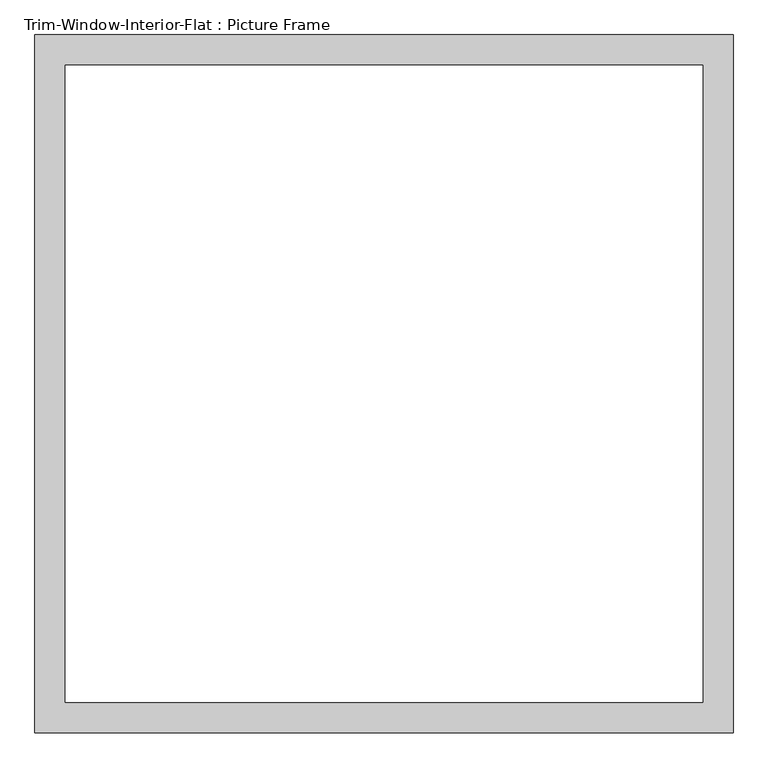
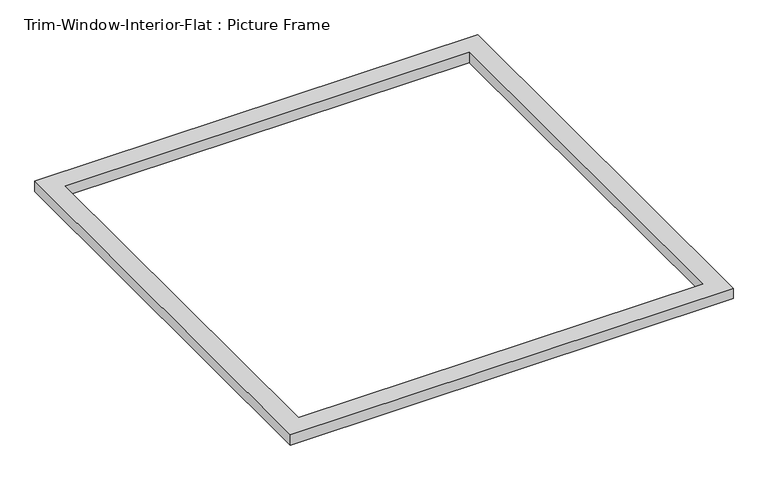
"""IFC4 building model written with IfcOpenShell, lengths in millimetres: proxy geometry, Trim-Window-Interior-Flat : Picture Frame."""

from ifc_helpers import new_model, si_unit, origin, origin_with_axes, place, context, project, spatial, polyline, outline, extrude, source, transform, mapped, element, save


def trim_window_interior_flat_picture_frame_caf2db4f(model_context):
    return source(origin(), model_context, "Body", "SweptSolid", [
        extrude(outline(polyline([(654.05, -44.45), (-654.05, -44.45), (-654.05, 1263.65), (654.05, 1263.65), (654.05, -44.45)]), holes=[polyline([(596.9, 12.7), (596.9, 1206.5), (-596.9, 1206.5), (-596.9, 12.7), (596.9, 12.7)])]), origin_with_axes(), (0.0, 0.0, 1.0), 31.75),
    ])


if __name__ == "__main__":
    model = new_model("IFC4")
    model_context = context("Model", 3, world=origin())
    ifc_project = project(units=[si_unit("LENGTHUNIT", "METRE", prefix="MILLI")], contexts=[model_context])
    site = spatial("IfcSite", under=ifc_project)
    building = spatial("IfcBuilding", under=site)
    placement = place(None, origin())
    trim_window_interior_flat_picture_frame_shape = trim_window_interior_flat_picture_frame_caf2db4f(model_context)
    element("IfcBuildingElementProxy", 1, Name="Trim-Window-Interior-Flat : Picture Frame", ObjectType="Trim-Window-Interior-Flat : Picture Frame", at=placement, inside=building, context=model_context, shape_type="MappedRepresentation", body=[
        mapped(trim_window_interior_flat_picture_frame_shape, transform((0.0, 0.0, 0.0), x_axis=(1.0, 0.0, 0.0), y_axis=(0.0, 1.0, 0.0), z_axis=(0.0, 0.0, 1.0))),
    ])
    save(model, "model.ifc")

# Revit data of these elements
# Type "Trim-Window-Interior-Flat : Picture Frame"
#   Trim Thickness_Picture Frame = 0' - 1 1/4"
#   Trim Width = 0' - 2 1/4"
#   Trim Thickness_with Sill = 0' - 0 3/4"
#   Sill Thickness = 0' - 1 1/4"
#   Opening Width [instance default] = 2' - 0"
#   Opening Height [instance default] = 3' - 0"
#   Default Elevation = 4' - 0"
#   Sill = no
#   Picture Frame = yes
#   Trim Material [instance default] = none
# Element 1 (IfcBuildingElementProxy, "Trim-Window-Interior-Flat : Picture Frame")
#   Opening Width = 4' - 0"
#   Opening Height = 4' - 0"
#   Trim Material = Wood - Stained
#   Materials on its faces: "Wood - Stained"
# Materials
#   "Wood - Stained": class "Wood", colour RGB 224 178 126, transparency 0, Cost = 0
